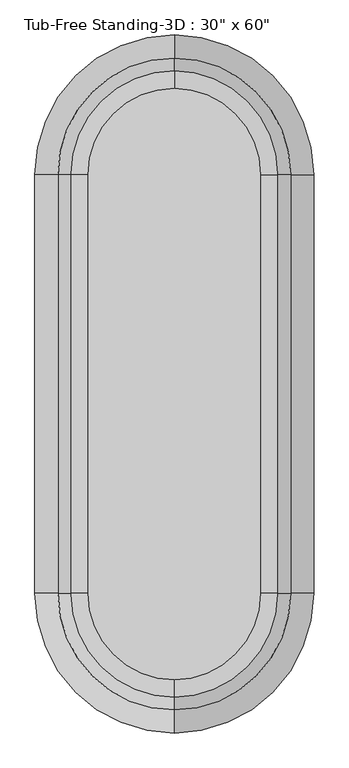
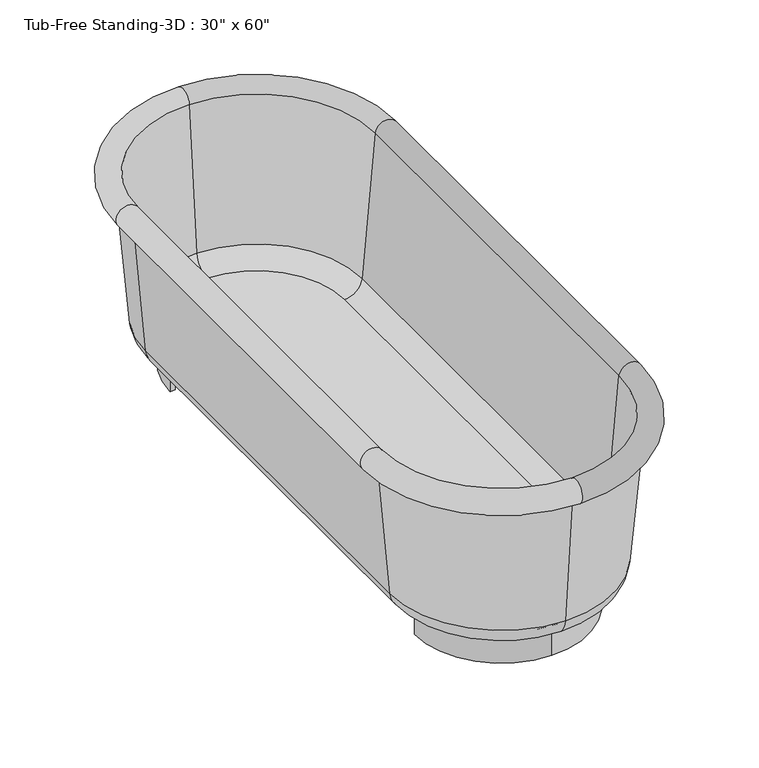
"""IFC4 building model written with IfcOpenShell, lengths in millimetres: flow terminal geometry."""

from ifc_helpers import new_model, si_unit, point, frame, frame_2d, origin, origin_with_axes, place, context, project, spatial, polyline, circle_curve, ellipse_curve, trimmed, segment, composite_curve, outline, extrude, source, transform, mapped, element, save
from ifc_brep_helpers import plane_surface, cylinder_surface, revolved_surface, advanced_brep


def flow_terminal_2ffd2f66(model_context):
    return source(origin(), model_context, "Body", "SolidModel", [
        extrude(outline(composite_curve([segment(trimmed(circle_curve(frame_2d((0.0, 457.2)), 177.8), [point((0.0, 635.0))], [point((-177.8, 457.2))], True, "CARTESIAN"), True, "CONTINUOUS"), segment(polyline([(-177.8, 457.2), (-188.0824236, 457.2)]), True, "CONTINUOUS"), segment(trimmed(circle_curve(frame_2d((0.0, 457.2)), 188.0824236), [point((-188.0824236, 457.2))], [point((0.0, 645.2824236))], False, "CARTESIAN"), True, "CONTINUOUS"), segment(trimmed(circle_curve(frame_2d((0.0, 457.2)), 188.0824236), [point((0.0, 645.2824236))], [point((188.0824236, 457.2))], False, "CARTESIAN"), True, "CONTINUOUS"), segment(polyline([(188.0824236, 457.2), (177.8, 457.2)]), True, "CONTINUOUS"), segment(trimmed(circle_curve(frame_2d((0.0, 457.2)), 177.8), [point((177.8, 457.2))], [point((0.0, 635.0))], True, "CARTESIAN"), True, "CONTINUOUS")], self_intersect=False)), origin_with_axes(), (0.0, 0.0, 1.0), 63.5),
        extrude(outline(composite_curve([segment(trimmed(circle_curve(frame_2d((0.0, -457.2)), 188.0824236), [point((0.0, -645.2824236))], [point((-188.0824236, -457.2))], False, "CARTESIAN"), True, "CONTINUOUS"), segment(polyline([(-188.0824236, -457.2), (-177.8, -457.2)]), True, "CONTINUOUS"), segment(trimmed(circle_curve(frame_2d((0.0, -457.2)), 177.8), [point((-177.8, -457.2))], [point((0.0, -635.0))], True, "CARTESIAN"), True, "CONTINUOUS"), segment(trimmed(circle_curve(frame_2d((0.0, -457.2)), 177.8), [point((0.0, -635.0))], [point((177.8, -457.2))], True, "CARTESIAN"), True, "CONTINUOUS"), segment(polyline([(177.8, -457.2), (188.0824236, -457.2)]), True, "CONTINUOUS"), segment(trimmed(circle_curve(frame_2d((0.0, -457.2)), 188.0824236), [point((188.0824236, -457.2))], [point((0.0, -645.2824236))], False, "CARTESIAN"), True, "CONTINUOUS")], self_intersect=False)), origin_with_axes(), (0.0, 0.0, 1.0), 63.5),
        extrude(outline(composite_curve([segment(polyline([(-188.0824236, -457.2), (-188.0824236, 457.2)]), True, "CONTINUOUS"), segment(trimmed(circle_curve(frame_2d((0.0, 457.2)), 188.0824236), [point((-188.0824236, 457.2))], [point((0.0, 645.2824236))], False, "CARTESIAN"), True, "CONTINUOUS"), segment(trimmed(circle_curve(frame_2d((0.0, 457.2)), 188.0824236), [point((0.0, 645.2824236))], [point((188.0824236, 457.2))], False, "CARTESIAN"), True, "CONTINUOUS"), segment(polyline([(188.0824236, 457.2), (188.0824236, -457.2)]), True, "CONTINUOUS"), segment(trimmed(circle_curve(frame_2d((0.0, -457.2)), 188.0824236), [point((188.0824236, -457.2))], [point((0.0, -645.2824236))], False, "CARTESIAN"), True, "CONTINUOUS"), segment(trimmed(circle_curve(frame_2d((0.0, -457.2)), 188.0824236), [point((0.0, -645.2824236))], [point((-188.0824236, -457.2))], False, "CARTESIAN"), True, "CONTINUOUS")], self_intersect=False)), frame((0.0, 0.0, 63.5), z_axis=(0.0, 0.0, 1.0), x_axis=(1.0, 0.0, 0.0)), (0.0, 0.0, 1.0), 15.08125),
        advanced_brep(
        [(0.0, -723.9, 406.4), (266.7, -457.2, 406.4), (279.4, -457.2, 406.4), (0.0, -736.6, 406.4), (0.0, -698.1045038, 111.5561295), (240.9045038, -457.2, 111.5561295), (0.0, -645.2824236, 63.1536107), (188.0824236, -457.2, 63.1536107), (0.0, -645.2824236, 78.0774627), (188.0824236, -457.2, 78.0774627), (0.0, -683.2374416, 112.8568289), (226.0374416, -457.2, 112.8568289), (0.0, -711.4561556, 435.3982063), (254.2561556, -457.2, 435.3982063), (-266.7, -457.2, 406.4), (-279.4, -457.2, 406.4), (-240.9045038, -457.2, 111.5561295), (-188.0824236, -457.2, 63.1536107), (-188.0824236, -457.2, 78.0774627), (-226.0374416, -457.2, 112.8568289), (-254.2561556, -457.2, 435.3982063), (-279.4, 457.2, 406.4), (-266.7, 457.2, 406.4), (-240.9045038, 457.2, 111.5561295), (-188.0824236, 457.2, 63.1536107), (-188.0824236, 457.2, 78.0774627), (-226.0374416, 457.2, 112.8568289), (-254.2561556, 457.2, 435.3982063), (0.0, 723.9, 406.4), (0.0, 736.6, 406.4), (0.0, 698.1045038, 111.5561295), (0.0, 645.2824236, 63.1536107), (0.0, 645.2824236, 78.0774627), (0.0, 683.2374416, 112.8568289), (0.0, 711.4561556, 435.3982063), (266.7, 457.2, 406.4), (279.4, 457.2, 406.4), (240.9045038, 457.2, 111.5561295), (188.0824236, 457.2, 63.1536107), (188.0824236, 457.2, 78.0774627), (226.0374416, 457.2, 112.8568289), (254.2561556, 457.2, 435.3982063)],
        [
            (0, 1, circle_curve(frame((0.0, -457.2, 406.4), z_axis=(0.0, 0.0, 1.0), x_axis=(1.0, 0.0, 0.0)), 266.7)),
            (1, 2),
            (2, 3, circle_curve(frame((0.0, -457.2, 406.4), z_axis=(0.0, 0.0, -1.0), x_axis=(1.0, 0.0, 0.0)), 279.4)),
            (3, 0),
            (4, 5, circle_curve(frame((0.0, -457.2, 111.5561295), z_axis=(0.0, 0.0, 1.0), x_axis=(1.0, 0.0, 0.0)), 240.9045038)),
            (5, 1),
            (0, 4),
            (6, 7, circle_curve(frame((0.0, -457.2, 63.1536107), z_axis=(0.0, 0.0, 1.0), x_axis=(1.0, 0.0, 0.0)), 188.0824236)),
            (7, 5, circle_curve(frame((188.0824236, -457.2, 116.1774627), z_axis=(0.0, -1.0, 0.0), x_axis=(1.0, 0.0, 0.0)), 53.023852)),
            (4, 6, circle_curve(frame((0.0, -645.2824236, 116.1774627), z_axis=(1.0, 0.0, 0.0), x_axis=(0.0, -1.0, 0.0)), 53.023852)),
            (8, 9, circle_curve(frame((0.0, -457.2, 78.0774627), z_axis=(0.0, 0.0, 1.0), x_axis=(1.0, 0.0, 0.0)), 188.0824236)),
            (9, 7),
            (6, 8),
            (10, 11, circle_curve(frame((0.0, -457.2, 112.8568289), z_axis=(0.0, 0.0, 1.0), x_axis=(1.0, 0.0, 0.0)), 226.0374416)),
            (11, 9, circle_curve(frame((188.0824236, -457.2, 116.1774627), z_axis=(0.0, 1.0, 0.0), x_axis=(1.0, 0.0, 0.0)), 38.1)),
            (8, 10, circle_curve(frame((0.0, -645.2824236, 116.1774627), z_axis=(-1.0, 0.0, 0.0), x_axis=(0.0, -1.0, 0.0)), 38.1)),
            (12, 13, circle_curve(frame((0.0, -457.2, 435.3982063), z_axis=(0.0, 0.0, 1.0), x_axis=(1.0, 0.0, 0.0)), 254.2561556)),
            (13, 11),
            (10, 12),
            (2, 13, circle_curve(frame((279.4, -457.2, 431.8), z_axis=(0.0, -1.0, 0.0), x_axis=(1.0, 0.0, 0.0)), 25.4)),
            (12, 3, circle_curve(frame((0.0, -736.6, 431.8), z_axis=(1.0, 0.0, 0.0), x_axis=(0.0, -1.0, 0.0)), 25.4)),
            (14, 0, circle_curve(frame((0.0, -457.2, 406.4), z_axis=(0.0, 0.0, 1.0), x_axis=(0.0, -1.0, 0.0)), 266.7)),
            (3, 15, circle_curve(frame((0.0, -457.2, 406.4), z_axis=(0.0, 0.0, -1.0), x_axis=(0.0, -1.0, 0.0)), 279.4)),
            (15, 14),
            (16, 4, circle_curve(frame((0.0, -457.2, 111.5561295), z_axis=(0.0, 0.0, 1.0), x_axis=(0.0, -1.0, 0.0)), 240.9045038)),
            (14, 16),
            (17, 6, circle_curve(frame((0.0, -457.2, 63.1536107), z_axis=(0.0, 0.0, 1.0), x_axis=(0.0, -1.0, 0.0)), 188.0824236)),
            (16, 17, circle_curve(frame((-188.0824236, -457.2, 116.1774627), z_axis=(0.0, -1.0, 0.0), x_axis=(-1.0, 0.0, 0.0)), 53.023852)),
            (18, 8, circle_curve(frame((0.0, -457.2, 78.0774627), z_axis=(0.0, 0.0, 1.0), x_axis=(0.0, -1.0, 0.0)), 188.0824236)),
            (17, 18),
            (19, 10, circle_curve(frame((0.0, -457.2, 112.8568289), z_axis=(0.0, 0.0, 1.0), x_axis=(0.0, -1.0, 0.0)), 226.0374416)),
            (18, 19, circle_curve(frame((-188.0824236, -457.2, 116.1774627), z_axis=(0.0, 1.0, 0.0), x_axis=(-1.0, 0.0, 0.0)), 38.1)),
            (20, 12, circle_curve(frame((0.0, -457.2, 435.3982063), z_axis=(0.0, 0.0, 1.0), x_axis=(0.0, -1.0, 0.0)), 254.2561556)),
            (19, 20),
            (20, 15, circle_curve(frame((-279.4, -457.2, 431.8), z_axis=(0.0, -1.0, 0.0), x_axis=(-1.0, 0.0, 0.0)), 25.4)),
            (15, 21),
            (21, 22),
            (22, 14),
            (22, 23),
            (23, 16),
            (23, 24, circle_curve(frame((-188.0824236, 457.2, 116.1774627), z_axis=(0.0, -1.0, 0.0), x_axis=(-1.0, 0.0, 0.0)), 53.023852)),
            (24, 17),
            (24, 25),
            (25, 18),
            (25, 26, circle_curve(frame((-188.0824236, 457.2, 116.1774627), z_axis=(0.0, 1.0, 0.0), x_axis=(-1.0, 0.0, 0.0)), 38.1)),
            (26, 19),
            (26, 27),
            (27, 20),
            (27, 21, circle_curve(frame((-279.4, 457.2, 431.8), z_axis=(0.0, -1.0, 0.0), x_axis=(-1.0, 0.0, 0.0)), 25.4)),
            (28, 22, circle_curve(frame((0.0, 457.2, 406.4), z_axis=(0.0, 0.0, 1.0), x_axis=(-1.0, 0.0, 0.0)), 266.7)),
            (21, 29, circle_curve(frame((0.0, 457.2, 406.4), z_axis=(0.0, 0.0, -1.0), x_axis=(-1.0, 0.0, 0.0)), 279.4)),
            (29, 28),
            (30, 23, circle_curve(frame((0.0, 457.2, 111.5561295), z_axis=(0.0, 0.0, 1.0), x_axis=(-1.0, 0.0, 0.0)), 240.9045038)),
            (28, 30),
            (31, 24, circle_curve(frame((0.0, 457.2, 63.1536107), z_axis=(0.0, 0.0, 1.0), x_axis=(-1.0, 0.0, 0.0)), 188.0824236)),
            (30, 31, circle_curve(frame((0.0, 645.2824236, 116.1774627), z_axis=(-1.0, 0.0, 0.0), x_axis=(0.0, 1.0, 0.0)), 53.023852)),
            (32, 25, circle_curve(frame((0.0, 457.2, 78.0774627), z_axis=(0.0, 0.0, 1.0), x_axis=(-1.0, 0.0, 0.0)), 188.0824236)),
            (31, 32),
            (33, 26, circle_curve(frame((0.0, 457.2, 112.8568289), z_axis=(0.0, 0.0, 1.0), x_axis=(-1.0, 0.0, 0.0)), 226.0374416)),
            (32, 33, circle_curve(frame((0.0, 645.2824236, 116.1774627), z_axis=(1.0, 0.0, 0.0), x_axis=(0.0, 1.0, 0.0)), 38.1)),
            (34, 27, circle_curve(frame((0.0, 457.2, 435.3982063), z_axis=(0.0, 0.0, 1.0), x_axis=(-1.0, 0.0, 0.0)), 254.2561556)),
            (33, 34),
            (34, 29, circle_curve(frame((0.0, 736.6, 431.8), z_axis=(-1.0, 0.0, 0.0), x_axis=(0.0, 1.0, 0.0)), 25.4)),
            (35, 28, circle_curve(frame((0.0, 457.2, 406.4), z_axis=(0.0, 0.0, 1.0), x_axis=(0.0, 1.0, 0.0)), 266.7)),
            (29, 36, circle_curve(frame((0.0, 457.2, 406.4), z_axis=(0.0, 0.0, -1.0), x_axis=(0.0, 1.0, 0.0)), 279.4)),
            (36, 35),
            (37, 30, circle_curve(frame((0.0, 457.2, 111.5561295), z_axis=(0.0, 0.0, 1.0), x_axis=(0.0, 1.0, 0.0)), 240.9045038)),
            (35, 37),
            (38, 31, circle_curve(frame((0.0, 457.2, 63.1536107), z_axis=(0.0, 0.0, 1.0), x_axis=(0.0, 1.0, 0.0)), 188.0824236)),
            (37, 38, circle_curve(frame((188.0824236, 457.2, 116.1774627), z_axis=(0.0, 1.0, 0.0), x_axis=(1.0, 0.0, 0.0)), 53.023852)),
            (39, 32, circle_curve(frame((0.0, 457.2, 78.0774627), z_axis=(0.0, 0.0, 1.0), x_axis=(0.0, 1.0, 0.0)), 188.0824236)),
            (38, 39),
            (40, 33, circle_curve(frame((0.0, 457.2, 112.8568289), z_axis=(0.0, 0.0, 1.0), x_axis=(0.0, 1.0, 0.0)), 226.0374416)),
            (39, 40, circle_curve(frame((188.0824236, 457.2, 116.1774627), z_axis=(0.0, -1.0, 0.0), x_axis=(1.0, 0.0, 0.0)), 38.1)),
            (41, 34, circle_curve(frame((0.0, 457.2, 435.3982063), z_axis=(0.0, 0.0, 1.0), x_axis=(0.0, 1.0, 0.0)), 254.2561556)),
            (40, 41),
            (41, 36, circle_curve(frame((279.4, 457.2, 431.8), z_axis=(0.0, 1.0, 0.0), x_axis=(1.0, 0.0, 0.0)), 25.4)),
            (36, 2),
            (1, 35),
            (5, 37),
            (7, 38),
            (9, 39),
            (11, 40),
            (13, 41),
        ],
        [
            plane_surface(frame((0.0, -457.2, 406.4), z_axis=(0.0, 0.0, -1.0), x_axis=(1.0, 0.0, 0.0))),
            revolved_surface(polyline([(266.7, -457.2, 406.4), (240.9045038, -457.2, 111.5561295)]), (0.0, -457.2, 431.8), (0.0, 0.0, -1.0)),
            revolved_surface(trimmed(ellipse_curve(frame((188.0824236, -457.2, 116.1774627), z_axis=(0.0, 1.0, 0.0), x_axis=(1.0, 0.0, 0.0)), 53.023852, 53.023852), [point((240.9045038, -457.2, 111.5561295))], [point((188.0824236, -457.2, 63.1536107))], True, "CARTESIAN"), (0.0, -457.2, 431.8), (0.0, 0.0, -1.0)),
            revolved_surface(polyline([(188.0824236, -457.2, 63.1536107), (188.0824236, -457.2, 78.07746270000001)]), (0.0, -457.2, 431.8), (0.0, 0.0, -1.0)),
            revolved_surface(trimmed(ellipse_curve(frame((188.0824236, -457.2, 116.1774627), z_axis=(0.0, -1.0, 0.0), x_axis=(1.0, 0.0, 0.0)), 38.1, 38.1), [point((188.0824236, -457.2, 78.0774627))], [point((226.0374416, -457.2, 112.8568289))], True, "CARTESIAN"), (0.0, -457.2, 431.8), (0.0, 0.0, -1.0)),
            revolved_surface(polyline([(226.0374416, -457.2, 112.8568289), (254.2561556, -457.2, 435.3982063)]), (0.0, -457.2, 431.8), (0.0, 0.0, -1.0)),
            revolved_surface(trimmed(ellipse_curve(frame((279.4, -457.2, 431.8), z_axis=(0.0, 1.0, 0.0), x_axis=(1.0, 0.0, 0.0)), 25.4, 25.4), [point((254.2561556, -457.2, 435.3982063))], [point((279.4, -457.2, 406.4))], True, "CARTESIAN"), (0.0, -457.2, 431.8), (0.0, 0.0, -1.0)),
            plane_surface(frame((0.0, -457.2, 406.4), z_axis=(0.0, 0.0, -1.0), x_axis=(0.0, -1.0, 0.0))),
            revolved_surface(polyline([(0.0, -723.9, 406.4), (0.0, -698.1045038, 111.5561295)]), (0.0, -457.2, 431.8), (0.0, 0.0, -1.0)),
            revolved_surface(trimmed(ellipse_curve(frame((0.0, -645.2824236, 116.1774627), z_axis=(1.0, 0.0, 0.0), x_axis=(0.0, -1.0, 0.0)), 53.023852, 53.023852), [point((0.0, -698.1045038, 111.5561295))], [point((0.0, -645.2824236, 63.1536107))], True, "CARTESIAN"), (0.0, -457.2, 431.8), (0.0, 0.0, -1.0)),
            revolved_surface(polyline([(0.0, -645.2824236, 63.1536107), (0.0, -645.2824236, 78.07746270000001)]), (0.0, -457.2, 431.8), (0.0, 0.0, -1.0)),
            revolved_surface(trimmed(ellipse_curve(frame((0.0, -645.2824236, 116.1774627), z_axis=(-1.0, 0.0, 0.0), x_axis=(0.0, -1.0, 0.0)), 38.1, 38.1), [point((0.0, -645.2824236, 78.0774627))], [point((0.0, -683.2374416, 112.8568289))], True, "CARTESIAN"), (0.0, -457.2, 431.8), (0.0, 0.0, -1.0)),
            revolved_surface(polyline([(0.0, -683.2374416, 112.8568289), (0.0, -711.4561556, 435.3982063)]), (0.0, -457.2, 431.8), (0.0, 0.0, -1.0)),
            revolved_surface(trimmed(ellipse_curve(frame((0.0, -736.6, 431.8), z_axis=(1.0, 0.0, 0.0), x_axis=(0.0, -1.0, 0.0)), 25.4, 25.4), [point((0.0, -711.4561556, 435.3982063))], [point((0.0, -736.6, 406.4))], True, "CARTESIAN"), (0.0, -457.2, 431.8), (0.0, 0.0, -1.0)),
            plane_surface(frame((-279.4, -457.2, 406.4), z_axis=(0.0, 0.0, -1.0), x_axis=(0.0, 1.0, 0.0))),
            plane_surface(frame((-266.7, -457.2, 406.4), z_axis=(-0.9961946980917455, 0.0, -0.08715574274765882), x_axis=(0.0, 1.0, 0.0))),
            cylinder_surface(frame((-188.0824236, -457.2, 116.1774627), z_axis=(0.0, -1.0, 0.0), x_axis=(-1.0, 0.0, 0.0)), 53.023852),
            plane_surface(frame((-188.0824236, -457.2, 63.1536107), z_axis=(1.0, 0.0, 0.0), x_axis=(0.0, 1.0, 0.0))),
            revolved_surface(polyline([(-226.1824236, 457.2, 116.1774627), (-226.1824236, -457.2, 116.1774627)]), (-188.0824236, -457.2, 116.1774627), (0.0, 1.0, 0.0)),
            plane_surface(frame((-226.0374416, -457.2, 112.8568289), z_axis=(0.9961946980917457, 0.0, 0.08715574274765679), x_axis=(0.0, 1.0, 0.0))),
            cylinder_surface(frame((-279.4, -457.2, 431.8), z_axis=(0.0, -1.0, 0.0), x_axis=(-1.0, 0.0, 0.0)), 25.4),
            plane_surface(frame((0.0, 457.2, 406.4), z_axis=(0.0, 0.0, -1.0), x_axis=(-1.0, 0.0, 0.0))),
            revolved_surface(polyline([(-266.7, 457.2, 406.4), (-240.9045038, 457.2, 111.5561295)]), (0.0, 457.2, 431.8), (0.0, 0.0, -1.0)),
            revolved_surface(trimmed(ellipse_curve(frame((-188.0824236, 457.2, 116.1774627), z_axis=(0.0, -1.0, 0.0), x_axis=(-1.0, 0.0, 0.0)), 53.023852, 53.023852), [point((-240.9045038, 457.2, 111.5561295))], [point((-188.0824236, 457.2, 63.1536107))], True, "CARTESIAN"), (0.0, 457.2, 431.8), (0.0, 0.0, -1.0)),
            revolved_surface(polyline([(-188.0824236, 457.2, 63.1536107), (-188.0824236, 457.2, 78.07746270000001)]), (0.0, 457.2, 431.8), (0.0, 0.0, -1.0)),
            revolved_surface(trimmed(ellipse_curve(frame((-188.0824236, 457.2, 116.1774627), z_axis=(0.0, 1.0, 0.0), x_axis=(-1.0, 0.0, 0.0)), 38.1, 38.1), [point((-188.0824236, 457.2, 78.0774627))], [point((-226.0374416, 457.2, 112.8568289))], True, "CARTESIAN"), (0.0, 457.2, 431.8), (0.0, 0.0, -1.0)),
            revolved_surface(polyline([(-226.0374416, 457.2, 112.8568289), (-254.2561556, 457.2, 435.3982063)]), (0.0, 457.2, 431.8), (0.0, 0.0, -1.0)),
            revolved_surface(trimmed(ellipse_curve(frame((-279.4, 457.2, 431.8), z_axis=(0.0, -1.0, 0.0), x_axis=(-1.0, 0.0, 0.0)), 25.4, 25.4), [point((-254.2561556, 457.2, 435.3982063))], [point((-279.4, 457.2, 406.4))], True, "CARTESIAN"), (0.0, 457.2, 431.8), (0.0, 0.0, -1.0)),
            plane_surface(frame((0.0, 457.2, 406.4), z_axis=(0.0, 0.0, -1.0), x_axis=(0.0, 1.0, 0.0))),
            revolved_surface(polyline([(0.0, 723.9, 406.4), (0.0, 698.1045038, 111.5561295)]), (0.0, 457.2, 431.8), (0.0, 0.0, -1.0)),
            revolved_surface(trimmed(ellipse_curve(frame((0.0, 645.2824236, 116.1774627), z_axis=(-1.0, 0.0, 0.0), x_axis=(0.0, 1.0, 0.0)), 53.023852, 53.023852), [point((0.0, 698.1045038, 111.5561295))], [point((0.0, 645.2824236, 63.1536107))], True, "CARTESIAN"), (0.0, 457.2, 431.8), (0.0, 0.0, -1.0)),
            revolved_surface(polyline([(0.0, 645.2824236, 63.1536107), (0.0, 645.2824236, 78.07746270000001)]), (0.0, 457.2, 431.8), (0.0, 0.0, -1.0)),
            revolved_surface(trimmed(ellipse_curve(frame((0.0, 645.2824236, 116.1774627), z_axis=(1.0, 0.0, 0.0), x_axis=(0.0, 1.0, 0.0)), 38.1, 38.1), [point((0.0, 645.2824236, 78.0774627))], [point((0.0, 683.2374416, 112.8568289))], True, "CARTESIAN"), (0.0, 457.2, 431.8), (0.0, 0.0, -1.0)),
            revolved_surface(polyline([(0.0, 683.2374416, 112.8568289), (0.0, 711.4561556, 435.3982063)]), (0.0, 457.2, 431.8), (0.0, 0.0, -1.0)),
            revolved_surface(trimmed(ellipse_curve(frame((0.0, 736.6, 431.8), z_axis=(-1.0, 0.0, 0.0), x_axis=(0.0, 1.0, 0.0)), 25.4, 25.4), [point((0.0, 711.4561556, 435.3982063))], [point((0.0, 736.6, 406.4))], True, "CARTESIAN"), (0.0, 457.2, 431.8), (0.0, 0.0, -1.0)),
            plane_surface(frame((279.4, 457.2, 406.4), z_axis=(0.0, 0.0, -1.0), x_axis=(0.0, -1.0, 0.0))),
            plane_surface(frame((266.7, 457.2, 406.4), z_axis=(0.9961946980917455, 0.0, -0.08715574274765882), x_axis=(0.0, -1.0, 0.0))),
            cylinder_surface(frame((188.0824236, 457.2, 116.1774627), z_axis=(0.0, 1.0, 0.0), x_axis=(1.0, 0.0, 0.0)), 53.023852),
            plane_surface(frame((188.0824236, 457.2, 63.1536107), z_axis=(-1.0, 0.0, 0.0), x_axis=(0.0, -1.0, 0.0))),
            revolved_surface(polyline([(226.1824236, -457.2, 116.1774627), (226.1824236, 457.2, 116.1774627)]), (188.0824236, 457.2, 116.1774627), (0.0, -1.0, 0.0)),
            plane_surface(frame((226.0374416, 457.2, 112.8568289), z_axis=(-0.9961946980917458, 0.0, 0.0871557427476568), x_axis=(0.0, -1.0, 0.0))),
            cylinder_surface(frame((279.4, 457.2, 431.8), z_axis=(0.0, 1.0, 0.0), x_axis=(1.0, 0.0, 0.0)), 25.4),
        ],
        [
            (0, [[1, 2, 3, 4]]),
            (1, [[5, 6, -1, 7]]),
            (2, [[8, 9, -5, 10]]),
            (3, [[11, 12, -8, 13]]),
            (4, [[14, 15, -11, 16]]),
            (5, [[17, 18, -14, 19]]),
            (6, [[-3, 20, -17, 21]]),
            (7, [[22, -4, 23, 24]]),
            (8, [[25, -7, -22, 26]]),
            (9, [[27, -10, -25, 28]]),
            (10, [[29, -13, -27, 30]]),
            (11, [[31, -16, -29, 32]]),
            (12, [[33, -19, -31, 34]]),
            (13, [[-23, -21, -33, 35]]),
            (14, [[-24, 36, 37, 38]]),
            (15, [[-26, -38, 39, 40]]),
            (16, [[-28, -40, 41, 42]]),
            (17, [[-30, -42, 43, 44]]),
            (18, [[-32, -44, 45, 46]]),
            (19, [[-34, -46, 47, 48]]),
            (20, [[-35, -48, 49, -36]]),
            (21, [[50, -37, 51, 52]]),
            (22, [[53, -39, -50, 54]]),
            (23, [[55, -41, -53, 56]]),
            (24, [[57, -43, -55, 58]]),
            (25, [[59, -45, -57, 60]]),
            (26, [[61, -47, -59, 62]]),
            (27, [[-51, -49, -61, 63]]),
            (28, [[64, -52, 65, 66]]),
            (29, [[67, -54, -64, 68]]),
            (30, [[69, -56, -67, 70]]),
            (31, [[71, -58, -69, 72]]),
            (32, [[73, -60, -71, 74]]),
            (33, [[75, -62, -73, 76]]),
            (34, [[-65, -63, -75, 77]]),
            (35, [[-66, 78, -2, 79]]),
            (36, [[-68, -79, -6, 80]]),
            (37, [[-70, -80, -9, 81]]),
            (38, [[-72, -81, -12, 82]]),
            (39, [[-74, -82, -15, 83]]),
            (40, [[-76, -83, -18, 84]]),
            (41, [[-77, -84, -20, -78]]),
        ],
    ),
    ])


if __name__ == "__main__":
    model = new_model("IFC4")
    model_context = context("Model", 3, world=origin())
    ifc_project = project(units=[si_unit("LENGTHUNIT", "METRE", prefix="MILLI")], contexts=[model_context])
    site = spatial("IfcSite", under=ifc_project)
    building = spatial("IfcBuilding", under=site)
    placement = place(None, origin())
    flow_terminal_shape = flow_terminal_2ffd2f66(model_context)
    element("IfcFlowTerminal", 1, ObjectType="Tub-Free Standing-3D : 30\" x 60\"", at=placement, inside=building, context=model_context, shape_type="MappedRepresentation", body=[
        mapped(flow_terminal_shape, transform((0.0, 0.0, 0.0), x_axis=(1.0, 0.0, 0.0), y_axis=(0.0, 1.0, 0.0), z_axis=(0.0, 0.0, 1.0))),
    ])
    save(model, "model.ifc")

# Revit data of these elements
# Type "Tub-Free Standing-3D : 30\" x 60\""
#   Assembly Code = "D2010110"
#   Height = 1' - 6"
#   Length = 5' - 0"
#   Width = 2' - 0"
#   Tub Material = Porcelain, Ivory
#   Default Elevation = 0
# Element 1 (IfcFlowTerminal, "Tub-Free Standing-3D : 30\" x 60\"")
#   Materials on its faces: "Porcelain, Ivory"
# Materials
#   "Porcelain, Ivory": class "Ceramic", colour RGB 247 247 239, transparency 0, Description = "Porcelain, ivory", Cost = 0
